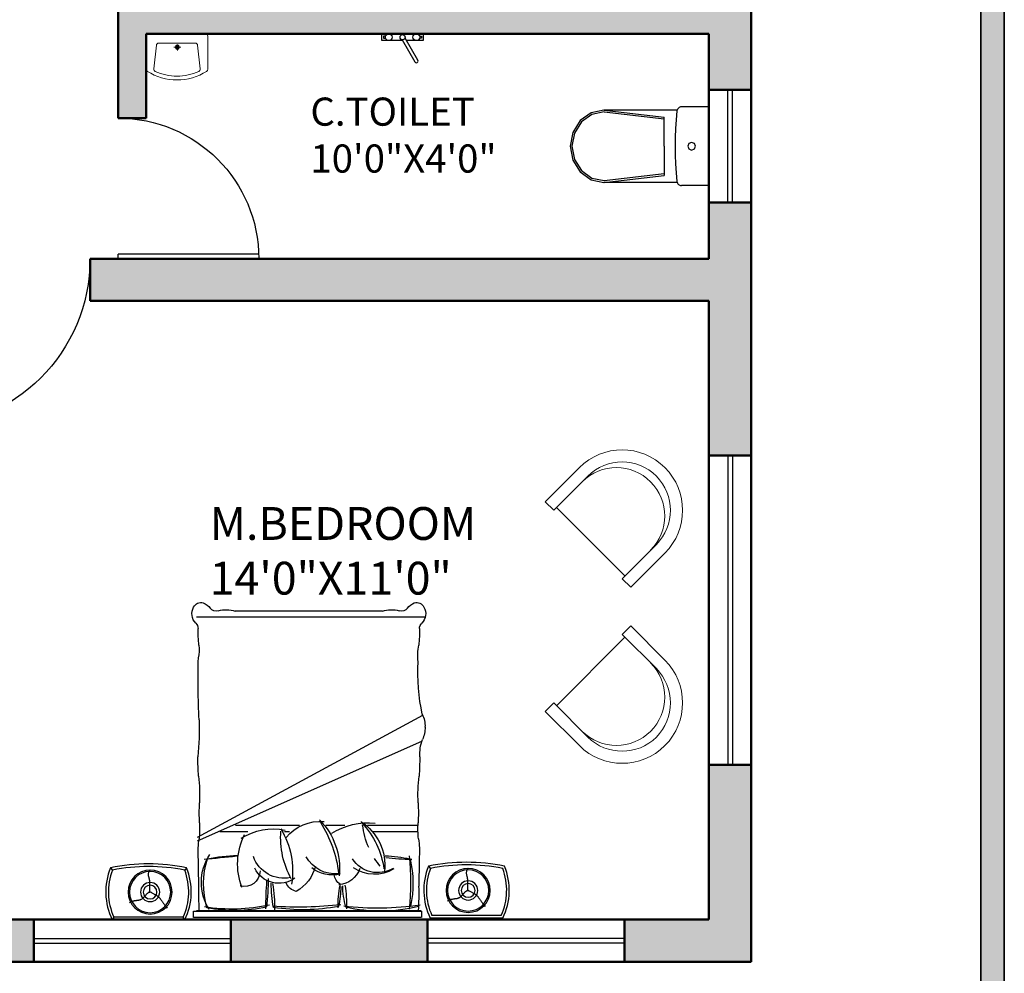
# Model space of a CAD drawing. Units: inches. Extents: x 3008 to 4088, y 1255 to 2137.
# Tile 9 of 30: x 3310 to 3520, y 1462 to 1665. Entities that reach past the tile are written whole.
import ezdxf

# ---------------------------------------------------------------- set-up
doc = ezdxf.new("R2010")
doc.units = ezdxf.units.IN
for name, color, linetype, lineweight in [('A-AREA-IDEN', 7, 'Continuous', 18), ('A-DOOR', 4, 'Continuous', 25), ('A-FLOR-FIXT', 8, 'Continuous', 18), ('A-FURN', 8, 'Continuous', 18), ('A-GLAZ', 4, 'Continuous', 25), ('A-WALL', 7, 'Continuous', 50), ('A-WALL-PATT', 8, 'Continuous', 13), ('C-PROP', 1, 'Continuous', 35), ('C-PROP-PATT', 9, 'Continuous', 13)]:
    doc.layers.add(name, color=color, linetype=linetype, lineweight=lineweight)
doc.layers.add('SANTEH', color=7, linetype='Continuous')
doc.layers.add('TEFRİŞ', color=11, linetype='Continuous')
doc.styles.get("Standard").update_dxf_attribs({"font": 'arial.ttf'})

# ---------------------------------------------------------------- blocks, each defined once
blk = doc.blocks.new('D2')
for p, q in [((1722.5, 1505.46), (1722.5, 1475.46)), ((1723.5, 1505.46), (1723.5, 1475.46)), ((1722.5, 1475.46), (1723.5, 1475.46))]:
    blk.add_line(p, q)
blk.add_arc((1722.5, 1475.46), 30, 0, 90)
blk = doc.blocks.new('D1')
for p, q in [((1805.96, 1500.36), (1805.96, 1464.36)), ((1806.96, 1500.36), (1806.96, 1464.36)), ((1805.96, 1464.36), (1806.96, 1464.36))]:
    blk.add_line(p, q)
blk.add_arc((1805.96, 1464.36), 36, 0, 90)
blk = doc.blocks.new('WC 2 Symb_109')
at = {"layer": 'SANTEH'}
for p, q in [((0, 0), (0, 380)), ((0, 380), (132.4, 380)), ((153.6, 364.9), (506.8, 364.9)), ((506.3, 364.9), (215.7, 330.9)), ((506.3, 356), (215.7, 322)), ((215.7, 190), (215.7, 330.9)), ((215.7, 190), (215.7, 49.1)), ((506.3, 24), (215.7, 58)), ((506.3, 15.1), (215.7, 49.1)), ((153.8, 15.1), (506.8, 15.1)), ((0, 0), (132.4, 0))]:
    blk.add_line(p, q, dxfattribs=at)
for points in [[(154.6, 360.1), (153.9, 364.1), (152.3, 367.9), (150.2, 371.3), (147.4, 374.3), (144.1, 376.7), (140.5, 378.5), (136.5, 379.6), (132.4, 380)], [(154.6, 19.7), (158.6, 62.1), (161.4, 104.7), (163.1, 147.3), (163.7, 189.9), (163.1, 232.5), (161.4, 275.1), (158.6, 317.7), (154.6, 360.1)], [(506.3, 24), (565.5, 36.6), (615.7, 72.6), (649.2, 126.5), (661, 190), (649.2, 253.5), (615.7, 307.4), (565.5, 343.4), (506.3, 356)], [(506.8, 15.1), (569.2, 28.4), (622.2, 66.3), (657.6, 123.1), (670, 190), (657.6, 256.9), (622.2, 313.7), (569.2, 351.6), (506.8, 364.9)], [(132.4, 0), (136.5, 0.4), (140.4, 1.5), (144.1, 3.2), (147.3, 5.6), (150.1, 8.6), (152.3, 12), (153.8, 15.7), (154.6, 19.7)]]:
    blk.add_lwpolyline(points, dxfattribs=at)
blk.add_lwpolyline([(83.6, 208.5), (70.4, 203.1), (64.9, 190), (70.4, 176.9), (83.6, 171.5), (96.8, 176.9), (102.2, 190), (96.8, 203.1)], close=True, dxfattribs=at)
blk = doc.blocks.new('Faucet - kit sink top')
at = {"layer": 'SANTEH'}
for p, q in [((-5.5, -0.75), (-5.5, -1.25)), ((-4.94278, -0.75), (-5.5, -0.75)), ((-5.5, -1.25), (-4.94278, -1.25)), ((-0.14775, -1.7441), (3.56698, -8.1782)), ((4.43301, -7.6782), (0.71828, -1.2441)), ((4.94278, -0.75), (5.5, -0.75)), ((5.5, -1.25), (4.94278, -1.25)), ((5.5, -0.75), (5.5, -1.25))]:
    blk.add_line(p, q, dxfattribs=at)
blk.add_lwpolyline([(-0.00587, -2), (-6, -2), (-6, 0), (6, 0), (6, -2), (1.15195, -2)], dxfattribs=at)
for centre, radius in [((-4, -1), 1), ((4, -1), 1), ((0, -1), 0.75)]:
    blk.add_circle(centre, radius, dxfattribs=at)
blk.add_arc((4, -7.9282), 0.5, 210, 30, dxfattribs=at)
blk = doc.blocks.new('A$C2EBB240D')
for p, q in [((0, 355.8), (0, 86.6)), ((480, 375.8), (20, 375.8)), ((500, 355.8), (500, 86.6)), ((60.8, 89.8), (82.3, 282.2)), ((250, 300), (102.1, 300)), ((250, 300), (397.9, 300)), ((439.2, 89.8), (417.7, 282.2))]:
    blk.add_line(p, q)
for points in [[(275.2, 266.4), (219.4, 266.4)], [(247.3, 238.5), (247.3, 288.9)]]:
    blk.add_lwpolyline(points)
for centre, radius, start, end in [((20, 355.8), 20, 90, 180), ((480, 355.8), 20, 0, 90), ((102.1, 280), 20, 90, 173.64284), ((247.3, 266.4), 16.7, 90, 270), ((247.3, 266.4), 10, 90, 270), ((247.3, 266.4), 16.7, 270, 90), ((247.3, 266.4), 10, 270, 90), ((397.9, 280), 20, 6.35716, 90), ((20, 86.6), 20, 180, 237.68921), ((80.7, 87.6), 20, 173.64284, 244.97956), ((419.3, 87.6), 20, 295.02044, 6.35716), ((480, 86.6), 20, 302.31079, 0), ((250, 450.3), 450.3, 237.68921, 270), ((250, 450.3), 420.3, 244.97956, 270), ((250, 450.3), 450.3, 270, 302.31079), ((250, 450.3), 420.3, 270, 295.02044)]:
    blk.add_arc(centre, radius, start, end)
blk = doc.blocks.new('12PSTG07')
at = {"color": 0, "linetype": 'ByBlock'}
for p, q in [((0, 15), (-12, 15)), ((0, 12), (0, 15)), ((-12, 12), (0, 12)), ((-1, -12), (-1, 12)), ((-12, -12), (0, -12)), ((0, -12), (0, -15)), ((0, -15), (-12, -15))]:
    blk.add_line(p, q, dxfattribs=at)
for centre, radius in [((-12, 0), 15), ((-12, 0), 12), ((-10, 0), 12)]:
    blk.add_arc(centre, radius, 90, 270, dxfattribs=at)
blk = doc.blocks.new('BED')
at = {"layer": 'TEFRİŞ'}
for p, q in [((2114.88, 1835.66), (2129.12, 1835.66)), ((2130.81, 1834.34), (2130.81, 1835.55)), ((2130.91, 1835.55), (2175.56, 1835.55)), ((2175.56, 1835.55), (2175.56, 1834.34)), ((2177.29, 1835.98), (2177.61, 1835.47)), ((2177.29, 1835.98), (2191.52, 1835.98)), ((2191.2, 1835.47), (2191.52, 1835.98)), ((2115.2, 1835.15), (2128.8, 1835.15)), ((2175.56, 1834.34), (2130.81, 1834.34)), ((2175, 1834.19), (2130.91, 1834.19)), ((2177.61, 1835.47), (2191.2, 1835.47)), ((2180.9, 1833.52), (2180.75, 1833.7)), ((2180.9, 1833.52), (2180.75, 1833.7)), ((2118.49, 1833.2), (2118.34, 1833.38)), ((2118.49, 1833.2), (2118.34, 1833.38)), ((2118.63, 1833.03), (2118.49, 1833.2)), ((2118.63, 1833.03), (2118.49, 1833.2)), ((2118.75, 1832.88), (2118.63, 1833.03)), ((2118.75, 1832.88), (2118.63, 1833.03)), ((2118.86, 1832.74), (2118.75, 1832.88)), ((2118.86, 1832.74), (2118.75, 1832.88)), ((2118.95, 1832.61), (2118.86, 1832.74)), ((2118.95, 1832.61), (2118.86, 1832.74)), ((2119.04, 1832.48), (2118.95, 1832.61)), ((2119.04, 1832.48), (2118.95, 1832.61)), ((2119.12, 1832.37), (2119.04, 1832.48)), ((2119.12, 1832.37), (2119.04, 1832.48)), ((2119.19, 1832.26), (2119.12, 1832.37)), ((2119.19, 1832.26), (2119.12, 1832.37)), ((2119.26, 1832.16), (2119.19, 1832.26)), ((2119.26, 1832.16), (2119.19, 1832.26)), ((2119.32, 1832.06), (2119.26, 1832.16)), ((2119.32, 1832.06), (2119.26, 1832.16)), ((2119.39, 1831.97), (2119.32, 1832.06)), ((2119.39, 1831.97), (2119.32, 1832.06)), ((2119.45, 1831.89), (2119.39, 1831.97)), ((2119.45, 1831.89), (2119.39, 1831.97)), ((2119.51, 1831.81), (2119.45, 1831.89)), ((2119.51, 1831.81), (2119.45, 1831.89)), ((2119.57, 1831.73), (2119.51, 1831.81)), ((2119.57, 1831.73), (2119.51, 1831.81)), ((2119.63, 1831.65), (2119.57, 1831.73)), ((2119.63, 1831.65), (2119.57, 1831.73)), ((2123.41, 1831.67), (2123.48, 1831.71)), ((2123.41, 1831.67), (2123.48, 1831.71)), ((2123.48, 1831.71), (2123.55, 1831.74)), ((2123.48, 1831.71), (2123.55, 1831.74)), ((2123.55, 1831.74), (2123.62, 1831.77)), ((2123.55, 1831.74), (2123.62, 1831.77)), ((2123.62, 1831.77), (2123.69, 1831.8)), ((2123.62, 1831.77), (2123.69, 1831.8)), ((2123.69, 1831.8), (2123.77, 1831.82)), ((2123.69, 1831.8), (2123.77, 1831.82)), ((2123.77, 1831.82), (2123.84, 1831.84)), ((2123.77, 1831.82), (2123.84, 1831.84)), ((2123.84, 1831.84), (2123.91, 1831.86)), ((2123.84, 1831.84), (2123.91, 1831.86)), ((2123.91, 1831.86), (2123.98, 1831.87)), ((2123.91, 1831.86), (2123.98, 1831.87)), ((2123.98, 1831.87), (2124.06, 1831.89)), ((2123.98, 1831.87), (2124.06, 1831.89)), ((2124.06, 1831.89), (2124.13, 1831.9)), ((2124.06, 1831.89), (2124.13, 1831.9)), ((2124.13, 1831.9), (2124.2, 1831.91)), ((2124.13, 1831.9), (2124.2, 1831.91)), ((2124.2, 1831.91), (2124.27, 1831.91)), ((2124.2, 1831.91), (2124.27, 1831.91)), ((2124.27, 1831.91), (2124.35, 1831.92)), ((2124.27, 1831.91), (2124.35, 1831.92)), ((2124.35, 1831.92), (2124.42, 1831.93)), ((2124.35, 1831.92), (2124.42, 1831.93)), ((2124.42, 1831.93), (2124.49, 1831.94)), ((2124.42, 1831.93), (2124.49, 1831.94)), ((2124.49, 1831.94), (2124.56, 1831.95)), ((2124.49, 1831.94), (2124.56, 1831.95)), ((2124.56, 1831.95), (2124.64, 1831.96)), ((2124.56, 1831.95), (2124.64, 1831.96)), ((2124.64, 1831.96), (2124.71, 1831.98)), ((2124.64, 1831.96), (2124.71, 1831.98)), ((2124.71, 1831.98), (2124.79, 1831.99)), ((2124.71, 1831.98), (2124.79, 1831.99)), ((2124.79, 1831.99), (2124.87, 1832.01)), ((2124.79, 1831.99), (2124.87, 1832.01)), ((2124.87, 1832.01), (2124.96, 1832.03)), ((2124.87, 1832.01), (2124.96, 1832.03)), ((2124.96, 1832.03), (2125.05, 1832.05)), ((2124.96, 1832.03), (2125.05, 1832.05)), ((2125.05, 1832.05), (2125.14, 1832.08)), ((2125.05, 1832.05), (2125.14, 1832.08)), ((2125.14, 1832.08), (2125.23, 1832.11)), ((2125.14, 1832.08), (2125.23, 1832.11)), ((2125.23, 1832.11), (2125.33, 1832.14)), ((2125.23, 1832.11), (2125.33, 1832.14)), ((2125.33, 1832.14), (2125.42, 1832.17)), ((2125.33, 1832.14), (2125.42, 1832.17)), ((2125.42, 1832.17), (2125.52, 1832.21)), ((2125.42, 1832.17), (2125.52, 1832.21)), ((2125.52, 1832.21), (2125.6, 1832.25)), ((2125.52, 1832.21), (2125.6, 1832.25)), ((2125.6, 1832.25), (2125.68, 1832.3)), ((2125.6, 1832.25), (2125.68, 1832.3)), ((2125.68, 1832.3), (2125.75, 1832.35)), ((2125.68, 1832.3), (2125.75, 1832.35)), ((2181.04, 1833.35), (2180.9, 1833.52)), ((2181.04, 1833.35), (2180.9, 1833.52)), ((2181.16, 1833.2), (2181.04, 1833.35)), ((2181.16, 1833.2), (2181.04, 1833.35)), ((2181.26, 1833.06), (2181.16, 1833.2)), ((2181.26, 1833.06), (2181.16, 1833.2)), ((2181.36, 1832.93), (2181.26, 1833.06)), ((2181.36, 1832.93), (2181.26, 1833.06)), ((2181.44, 1832.8), (2181.36, 1832.93)), ((2181.44, 1832.8), (2181.36, 1832.93)), ((2181.52, 1832.69), (2181.44, 1832.8)), ((2181.52, 1832.69), (2181.44, 1832.8)), ((2181.59, 1832.58), (2181.52, 1832.69)), ((2181.59, 1832.58), (2181.52, 1832.69)), ((2181.66, 1832.48), (2181.59, 1832.58)), ((2181.66, 1832.48), (2181.59, 1832.58)), ((2181.73, 1832.38), (2181.66, 1832.48)), ((2181.73, 1832.38), (2181.66, 1832.48)), ((2181.79, 1832.29), (2181.73, 1832.38)), ((2181.79, 1832.29), (2181.73, 1832.38)), ((2181.85, 1832.21), (2181.79, 1832.29)), ((2181.85, 1832.21), (2181.79, 1832.29)), ((2181.92, 1832.13), (2181.85, 1832.21)), ((2181.92, 1832.13), (2181.85, 1832.21)), ((2181.97, 1832.05), (2181.92, 1832.13)), ((2181.97, 1832.05), (2181.92, 1832.13)), ((2182.03, 1831.97), (2181.97, 1832.05)), ((2182.03, 1831.97), (2181.97, 1832.05)), ((2182.09, 1831.9), (2182.03, 1831.97)), ((2182.09, 1831.9), (2182.03, 1831.97)), ((2182.15, 1831.83), (2182.09, 1831.9)), ((2182.15, 1831.83), (2182.09, 1831.9)), ((2182.21, 1831.76), (2182.15, 1831.83)), ((2182.21, 1831.76), (2182.15, 1831.83)), ((2182.27, 1831.7), (2182.21, 1831.76)), ((2182.27, 1831.7), (2182.21, 1831.76)), ((2182.33, 1831.63), (2182.27, 1831.7)), ((2182.33, 1831.63), (2182.27, 1831.7)), ((2185.42, 1831.65), (2185.48, 1831.72)), ((2185.42, 1831.65), (2185.48, 1831.72)), ((2185.48, 1831.72), (2185.55, 1831.78)), ((2185.48, 1831.72), (2185.55, 1831.78)), ((2185.55, 1831.78), (2185.61, 1831.84)), ((2185.55, 1831.78), (2185.61, 1831.84)), ((2185.61, 1831.84), (2185.68, 1831.9)), ((2185.61, 1831.84), (2185.68, 1831.9)), ((2185.68, 1831.9), (2185.75, 1831.95)), ((2185.68, 1831.9), (2185.75, 1831.95)), ((2185.75, 1831.95), (2185.82, 1831.99)), ((2185.75, 1831.95), (2185.82, 1831.99)), ((2185.82, 1831.99), (2185.89, 1832.03)), ((2185.82, 1831.99), (2185.89, 1832.03)), ((2185.89, 1832.03), (2185.96, 1832.06)), ((2185.89, 1832.03), (2185.96, 1832.06)), ((2185.96, 1832.06), (2186.03, 1832.09)), ((2185.96, 1832.06), (2186.03, 1832.09)), ((2186.03, 1832.09), (2186.1, 1832.12)), ((2186.03, 1832.09), (2186.1, 1832.12)), ((2186.1, 1832.12), (2186.17, 1832.14)), ((2186.1, 1832.12), (2186.17, 1832.14)), ((2186.17, 1832.14), (2186.24, 1832.16)), ((2186.17, 1832.14), (2186.24, 1832.16)), ((2186.24, 1832.16), (2186.32, 1832.18)), ((2186.24, 1832.16), (2186.32, 1832.18)), ((2186.32, 1832.18), (2186.39, 1832.19)), ((2186.32, 1832.18), (2186.39, 1832.19)), ((2186.39, 1832.19), (2186.46, 1832.21)), ((2186.39, 1832.19), (2186.46, 1832.21)), ((2186.46, 1832.21), (2186.53, 1832.22)), ((2186.46, 1832.21), (2186.53, 1832.22)), ((2186.53, 1832.22), (2186.61, 1832.23)), ((2186.53, 1832.22), (2186.61, 1832.23)), ((2186.61, 1832.23), (2186.68, 1832.23)), ((2186.61, 1832.23), (2186.68, 1832.23)), ((2186.68, 1832.23), (2186.75, 1832.24)), ((2186.68, 1832.23), (2186.75, 1832.24)), ((2186.75, 1832.24), (2186.82, 1832.25)), ((2186.75, 1832.24), (2186.82, 1832.25)), ((2186.82, 1832.25), (2186.9, 1832.26)), ((2186.82, 1832.25), (2186.9, 1832.26)), ((2186.9, 1832.26), (2186.97, 1832.27)), ((2186.9, 1832.26), (2186.97, 1832.27)), ((2186.97, 1832.27), (2187.04, 1832.28)), ((2186.97, 1832.27), (2187.04, 1832.28)), ((2187.04, 1832.28), (2187.12, 1832.3)), ((2187.04, 1832.28), (2187.12, 1832.3)), ((2187.12, 1832.3), (2187.2, 1832.31)), ((2187.12, 1832.3), (2187.2, 1832.31)), ((2187.2, 1832.31), (2187.28, 1832.33)), ((2187.2, 1832.31), (2187.28, 1832.33)), ((2187.28, 1832.33), (2187.36, 1832.35)), ((2187.28, 1832.33), (2187.36, 1832.35)), ((2187.36, 1832.35), (2187.45, 1832.37)), ((2187.36, 1832.35), (2187.45, 1832.37)), ((2187.45, 1832.37), (2187.54, 1832.4)), ((2187.45, 1832.37), (2187.54, 1832.4)), ((2187.54, 1832.4), (2187.64, 1832.43)), ((2187.54, 1832.4), (2187.64, 1832.43)), ((2187.64, 1832.43), (2187.74, 1832.46)), ((2187.64, 1832.43), (2187.74, 1832.46)), ((2187.74, 1832.46), (2187.83, 1832.49)), ((2187.74, 1832.46), (2187.83, 1832.49)), ((2187.83, 1832.49), (2187.92, 1832.53)), ((2187.83, 1832.49), (2187.92, 1832.53)), ((2187.92, 1832.53), (2188.01, 1832.57)), ((2187.92, 1832.53), (2188.01, 1832.57)), ((2188.01, 1832.57), (2188.09, 1832.62)), ((2188.01, 1832.57), (2188.09, 1832.62)), ((2188.09, 1832.62), (2188.15, 1832.67)), ((2188.09, 1832.62), (2188.15, 1832.67)), ((2119.69, 1831.58), (2119.63, 1831.65)), ((2119.69, 1831.58), (2119.63, 1831.65)), ((2119.75, 1831.51), (2119.69, 1831.58)), ((2119.75, 1831.51), (2119.69, 1831.58)), ((2119.81, 1831.44), (2119.75, 1831.51)), ((2119.81, 1831.44), (2119.75, 1831.51)), ((2119.87, 1831.38), (2119.81, 1831.44)), ((2119.87, 1831.38), (2119.81, 1831.44)), ((2119.93, 1831.31), (2119.87, 1831.38)), ((2119.93, 1831.31), (2119.87, 1831.38)), ((2119.99, 1831.25), (2119.93, 1831.31)), ((2119.99, 1831.25), (2119.93, 1831.31)), ((2120.05, 1831.2), (2119.99, 1831.25)), ((2120.05, 1831.2), (2119.99, 1831.25)), ((2120.12, 1831.14), (2120.05, 1831.2)), ((2120.12, 1831.14), (2120.05, 1831.2)), ((2120.18, 1831.09), (2120.12, 1831.14)), ((2120.18, 1831.09), (2120.12, 1831.14)), ((2120.25, 1831.04), (2120.18, 1831.09)), ((2120.25, 1831.04), (2120.18, 1831.09)), ((2120.32, 1830.99), (2120.25, 1831.04)), ((2120.32, 1830.99), (2120.25, 1831.04)), ((2120.39, 1830.94), (2120.32, 1830.99)), ((2120.39, 1830.94), (2120.32, 1830.99)), ((2120.47, 1830.9), (2120.39, 1830.94)), ((2120.47, 1830.9), (2120.39, 1830.94)), ((2120.54, 1830.85), (2120.47, 1830.9)), ((2120.54, 1830.85), (2120.47, 1830.9)), ((2120.62, 1830.8), (2120.54, 1830.85)), ((2120.62, 1830.8), (2120.54, 1830.85)), ((2120.7, 1830.75), (2120.62, 1830.8)), ((2120.7, 1830.75), (2120.62, 1830.8)), ((2120.79, 1830.7), (2120.7, 1830.75)), ((2120.79, 1830.7), (2120.7, 1830.75)), ((2120.88, 1830.65), (2120.79, 1830.7)), ((2120.88, 1830.65), (2120.79, 1830.7)), ((2120.98, 1830.59), (2120.88, 1830.65)), ((2120.98, 1830.59), (2120.88, 1830.65)), ((2121.09, 1830.52), (2120.98, 1830.59)), ((2121.09, 1830.52), (2120.98, 1830.59)), ((2121.21, 1830.45), (2121.09, 1830.52)), ((2121.21, 1830.45), (2121.09, 1830.52)), ((2121.34, 1830.38), (2121.21, 1830.45)), ((2121.34, 1830.38), (2121.21, 1830.45)), ((2121.49, 1830.29), (2121.34, 1830.38)), ((2121.49, 1830.29), (2121.34, 1830.38)), ((2121.66, 1830.21), (2121.49, 1830.29)), ((2121.66, 1830.21), (2121.49, 1830.29)), ((2121.66, 1830.18), (2121.87, 1830.29)), ((2121.66, 1830.18), (2121.87, 1830.29)), ((2121.85, 1830.11), (2121.66, 1830.21)), ((2121.85, 1830.11), (2121.66, 1830.21)), ((2121.74, 1829.99), (2121.73, 1829.83)), ((2121.74, 1829.99), (2121.73, 1829.83)), ((2121.73, 1829.83), (2121.73, 1829.69)), ((2121.73, 1829.83), (2121.73, 1829.69)), ((2121.76, 1830.38), (2121.74, 1830.17)), ((2121.76, 1830.38), (2121.74, 1830.17)), ((2121.74, 1830.17), (2121.74, 1829.99)), ((2121.74, 1830.17), (2121.74, 1829.99)), ((2121.87, 1830.29), (2122.04, 1830.4)), ((2121.87, 1830.29), (2122.04, 1830.4)), ((2122.04, 1830.4), (2122.2, 1830.51)), ((2122.04, 1830.4), (2122.2, 1830.51)), ((2122.2, 1830.51), (2122.33, 1830.61)), ((2122.2, 1830.51), (2122.33, 1830.61)), ((2122.33, 1830.61), (2122.45, 1830.72)), ((2122.33, 1830.61), (2122.45, 1830.72)), ((2122.45, 1830.72), (2122.55, 1830.82)), ((2122.45, 1830.72), (2122.55, 1830.82)), ((2122.55, 1830.82), (2122.64, 1830.91)), ((2122.55, 1830.82), (2122.64, 1830.91)), ((2122.64, 1830.91), (2122.72, 1831.01)), ((2122.64, 1830.91), (2122.72, 1831.01)), ((2122.72, 1831.01), (2122.8, 1831.09)), ((2122.72, 1831.01), (2122.8, 1831.09)), ((2122.8, 1831.09), (2122.87, 1831.18)), ((2122.8, 1831.09), (2122.87, 1831.18)), ((2122.87, 1831.18), (2122.94, 1831.26)), ((2122.87, 1831.18), (2122.94, 1831.26)), ((2122.94, 1831.26), (2123.01, 1831.33)), ((2122.94, 1831.26), (2123.01, 1831.33)), ((2123.01, 1831.33), (2123.08, 1831.4)), ((2123.01, 1831.33), (2123.08, 1831.4)), ((2123.08, 1831.4), (2123.14, 1831.46)), ((2123.08, 1831.4), (2123.14, 1831.46)), ((2123.14, 1831.46), (2123.21, 1831.52)), ((2123.14, 1831.46), (2123.21, 1831.52)), ((2123.21, 1831.52), (2123.27, 1831.58)), ((2123.21, 1831.52), (2123.27, 1831.58)), ((2123.27, 1831.58), (2123.34, 1831.63)), ((2123.27, 1831.58), (2123.34, 1831.63)), ((2123.34, 1831.63), (2123.41, 1831.67)), ((2123.34, 1831.63), (2123.41, 1831.67)), ((2182.4, 1831.57), (2182.33, 1831.63)), ((2182.4, 1831.57), (2182.33, 1831.63)), ((2182.46, 1831.52), (2182.4, 1831.57)), ((2182.46, 1831.52), (2182.4, 1831.57)), ((2182.52, 1831.46), (2182.46, 1831.52)), ((2182.52, 1831.46), (2182.46, 1831.52)), ((2182.59, 1831.41), (2182.52, 1831.46)), ((2182.59, 1831.41), (2182.52, 1831.46)), ((2182.66, 1831.36), (2182.59, 1831.41)), ((2182.66, 1831.36), (2182.59, 1831.41)), ((2182.73, 1831.31), (2182.66, 1831.36)), ((2182.73, 1831.31), (2182.66, 1831.36)), ((2182.8, 1831.26), (2182.73, 1831.31)), ((2182.8, 1831.26), (2182.73, 1831.31)), ((2182.87, 1831.22), (2182.8, 1831.26)), ((2182.87, 1831.22), (2182.8, 1831.26)), ((2182.95, 1831.17), (2182.87, 1831.22)), ((2182.95, 1831.17), (2182.87, 1831.22)), ((2183.03, 1831.12), (2182.95, 1831.17)), ((2183.03, 1831.12), (2182.95, 1831.17)), ((2183.11, 1831.07), (2183.03, 1831.12)), ((2183.11, 1831.07), (2183.03, 1831.12)), ((2183.2, 1831.02), (2183.11, 1831.07)), ((2183.2, 1831.02), (2183.11, 1831.07)), ((2183.29, 1830.97), (2183.2, 1831.02)), ((2183.29, 1830.97), (2183.2, 1831.02)), ((2183.39, 1830.91), (2183.29, 1830.97)), ((2183.39, 1830.91), (2183.29, 1830.97)), ((2183.49, 1830.84), (2183.39, 1830.91)), ((2183.49, 1830.84), (2183.39, 1830.91)), ((2183.61, 1830.77), (2183.49, 1830.84)), ((2183.61, 1830.77), (2183.49, 1830.84)), ((2183.75, 1830.7), (2183.61, 1830.77)), ((2183.75, 1830.7), (2183.61, 1830.77)), ((2183.9, 1830.61), (2183.75, 1830.7)), ((2183.9, 1830.61), (2183.75, 1830.7)), ((2184.06, 1830.53), (2183.9, 1830.61)), ((2184.06, 1830.53), (2183.9, 1830.61)), ((2184.25, 1830.43), (2184.06, 1830.53)), ((2184.25, 1830.43), (2184.06, 1830.53)), ((2184.07, 1830.5), (2184.27, 1830.61)), ((2184.07, 1830.5), (2184.27, 1830.61)), ((2184.15, 1830.49), (2184.14, 1830.31)), ((2184.15, 1830.49), (2184.14, 1830.31)), ((2184.14, 1830.31), (2184.14, 1830.15)), ((2184.14, 1830.31), (2184.14, 1830.15)), ((2184.14, 1830.15), (2184.14, 1830.01)), ((2184.14, 1830.15), (2184.14, 1830.01)), ((2184.14, 1830.01), (2184.14, 1829.89)), ((2184.14, 1830.01), (2184.14, 1829.89)), ((2184.14, 1829.89), (2184.14, 1829.77)), ((2184.14, 1829.89), (2184.14, 1829.77)), ((2184.14, 1829.77), (2184.14, 1829.67)), ((2184.14, 1829.77), (2184.14, 1829.67)), ((2184.17, 1830.7), (2184.15, 1830.49)), ((2184.17, 1830.7), (2184.15, 1830.49)), ((2184.27, 1830.61), (2184.45, 1830.72)), ((2184.27, 1830.61), (2184.45, 1830.72)), ((2184.45, 1830.72), (2184.6, 1830.83)), ((2184.45, 1830.72), (2184.6, 1830.83)), ((2184.6, 1830.83), (2184.74, 1830.93)), ((2184.6, 1830.83), (2184.74, 1830.93)), ((2184.74, 1830.93), (2184.85, 1831.04)), ((2184.74, 1830.93), (2184.85, 1831.04)), ((2184.85, 1831.04), (2184.95, 1831.14)), ((2184.85, 1831.04), (2184.95, 1831.14)), ((2184.95, 1831.14), (2185.05, 1831.23)), ((2184.95, 1831.14), (2185.05, 1831.23)), ((2185.05, 1831.23), (2185.13, 1831.33)), ((2185.05, 1831.23), (2185.13, 1831.33)), ((2185.13, 1831.33), (2185.21, 1831.41)), ((2185.13, 1831.33), (2185.21, 1831.41)), ((2185.21, 1831.41), (2185.28, 1831.5)), ((2185.21, 1831.41), (2185.28, 1831.5)), ((2185.28, 1831.5), (2185.35, 1831.58)), ((2185.28, 1831.5), (2185.35, 1831.58)), ((2185.35, 1831.58), (2185.42, 1831.65)), ((2185.35, 1831.58), (2185.42, 1831.65)), ((2121.73, 1829.69), (2121.73, 1829.57)), ((2121.73, 1829.69), (2121.73, 1829.57)), ((2121.73, 1829.57), (2121.73, 1829.45)), ((2121.73, 1829.57), (2121.73, 1829.45)), ((2121.73, 1829.45), (2121.74, 1829.35)), ((2121.73, 1829.45), (2121.74, 1829.35)), ((2121.74, 1828.89), (2121.73, 1828.8)), ((2121.74, 1828.89), (2121.73, 1828.8)), ((2121.73, 1828.8), (2121.73, 1828.72)), ((2121.73, 1828.8), (2121.73, 1828.72)), ((2121.73, 1828.72), (2121.73, 1828.64)), ((2121.73, 1828.72), (2121.73, 1828.64)), ((2121.73, 1828.64), (2121.73, 1828.56)), ((2121.73, 1828.64), (2121.73, 1828.56)), ((2121.73, 1828.56), (2121.73, 1828.48)), ((2121.73, 1828.56), (2121.73, 1828.48)), ((2121.73, 1828.48), (2121.73, 1828.4)), ((2121.73, 1828.48), (2121.73, 1828.4)), ((2121.73, 1828.4), (2121.73, 1828.33)), ((2121.73, 1828.4), (2121.73, 1828.33)), ((2121.73, 1828.33), (2121.74, 1828.25)), ((2121.73, 1828.33), (2121.74, 1828.25)), ((2121.74, 1829.35), (2121.74, 1829.25)), ((2121.74, 1829.35), (2121.74, 1829.25)), ((2121.74, 1829.25), (2121.74, 1829.16)), ((2121.74, 1829.25), (2121.74, 1829.16)), ((2121.74, 1829.16), (2121.74, 1829.06)), ((2121.74, 1829.16), (2121.74, 1829.06)), ((2121.74, 1829.06), (2121.74, 1828.97)), ((2121.74, 1829.06), (2121.74, 1828.97)), ((2121.74, 1828.97), (2121.74, 1828.89)), ((2121.74, 1828.97), (2121.74, 1828.89)), ((2121.74, 1828.25), (2121.75, 1828.18)), ((2121.74, 1828.25), (2121.75, 1828.18)), ((2121.75, 1828.18), (2121.75, 1828.1)), ((2121.75, 1828.18), (2121.75, 1828.1)), ((2121.75, 1828.1), (2121.76, 1828.03)), ((2121.75, 1828.1), (2121.76, 1828.03)), ((2121.76, 1828.03), (2121.78, 1827.95)), ((2121.76, 1828.03), (2121.78, 1827.95)), ((2121.78, 1827.95), (2121.79, 1827.88)), ((2121.78, 1827.95), (2121.79, 1827.88)), ((2121.79, 1827.88), (2121.8, 1827.8)), ((2121.79, 1827.88), (2121.8, 1827.8)), ((2184.14, 1829.04), (2184.13, 1828.96)), ((2184.14, 1829.04), (2184.13, 1828.96)), ((2184.13, 1828.96), (2184.13, 1828.88)), ((2184.13, 1828.96), (2184.13, 1828.88)), ((2184.13, 1828.88), (2184.13, 1828.8)), ((2184.13, 1828.88), (2184.13, 1828.8)), ((2184.13, 1828.8), (2184.14, 1828.72)), ((2184.13, 1828.8), (2184.14, 1828.72)), ((2184.14, 1829.67), (2184.15, 1829.57)), ((2184.14, 1829.67), (2184.15, 1829.57)), ((2184.15, 1829.38), (2184.14, 1829.29)), ((2184.15, 1829.38), (2184.14, 1829.29)), ((2184.14, 1829.29), (2184.14, 1829.21)), ((2184.14, 1829.29), (2184.14, 1829.21)), ((2184.14, 1829.21), (2184.14, 1829.12)), ((2184.14, 1829.21), (2184.14, 1829.12)), ((2184.14, 1829.12), (2184.14, 1829.04)), ((2184.14, 1829.12), (2184.14, 1829.04)), ((2184.14, 1828.72), (2184.14, 1828.65)), ((2184.14, 1828.72), (2184.14, 1828.65)), ((2184.14, 1828.65), (2184.15, 1828.57)), ((2184.14, 1828.65), (2184.15, 1828.57)), ((2184.15, 1829.57), (2184.15, 1829.48)), ((2184.15, 1829.57), (2184.15, 1829.48)), ((2184.15, 1829.48), (2184.15, 1829.38)), ((2184.15, 1829.48), (2184.15, 1829.38)), ((2184.15, 1828.57), (2184.15, 1828.5)), ((2184.15, 1828.57), (2184.15, 1828.5)), ((2184.15, 1828.5), (2184.16, 1828.42)), ((2184.15, 1828.5), (2184.16, 1828.42)), ((2184.16, 1828.42), (2184.17, 1828.35)), ((2184.16, 1828.42), (2184.17, 1828.35)), ((2184.17, 1828.35), (2184.18, 1828.27)), ((2184.17, 1828.35), (2184.18, 1828.27)), ((2184.18, 1828.27), (2184.19, 1828.2)), ((2184.18, 1828.27), (2184.19, 1828.2)), ((2184.19, 1828.2), (2184.21, 1828.12)), ((2184.19, 1828.2), (2184.21, 1828.12)), ((2184.21, 1828.12), (2184.22, 1828.04)), ((2184.21, 1828.12), (2184.22, 1828.04)), ((2184.22, 1828.04), (2184.24, 1827.97)), ((2184.22, 1828.04), (2184.24, 1827.97)), ((2184.24, 1827.97), (2184.26, 1827.89)), ((2184.24, 1827.97), (2184.26, 1827.89)), ((2184.26, 1827.89), (2184.28, 1827.81)), ((2184.26, 1827.89), (2184.28, 1827.81)), ((2184.28, 1827.81), (2184.3, 1827.73)), ((2184.28, 1827.81), (2184.3, 1827.73)), ((2121.78, 1825.93), (2121.74, 1825.8)), ((2121.78, 1825.93), (2121.74, 1825.8)), ((2121.83, 1826.06), (2121.78, 1825.93)), ((2121.83, 1826.06), (2121.78, 1825.93)), ((2121.8, 1827.8), (2121.82, 1827.72)), ((2121.8, 1827.8), (2121.82, 1827.72)), ((2121.82, 1827.72), (2121.84, 1827.65)), ((2121.82, 1827.72), (2121.84, 1827.65)), ((2121.87, 1826.19), (2121.83, 1826.06)), ((2121.87, 1826.19), (2121.83, 1826.06)), ((2121.84, 1827.65), (2121.85, 1827.57)), ((2121.84, 1827.65), (2121.85, 1827.57)), ((2121.85, 1827.57), (2121.87, 1827.49)), ((2121.85, 1827.57), (2121.87, 1827.49)), ((2121.87, 1827.49), (2121.89, 1827.41)), ((2121.87, 1827.49), (2121.89, 1827.41)), ((2121.91, 1826.31), (2121.87, 1826.19)), ((2121.91, 1826.31), (2121.87, 1826.19)), ((2121.89, 1827.41), (2121.91, 1827.33)), ((2121.89, 1827.41), (2121.91, 1827.33)), ((2121.91, 1827.33), (2121.93, 1827.26)), ((2121.91, 1827.33), (2121.93, 1827.26)), ((2121.95, 1826.42), (2121.91, 1826.31)), ((2121.95, 1826.42), (2121.91, 1826.31)), ((2121.93, 1827.26), (2121.95, 1827.18)), ((2121.93, 1827.26), (2121.95, 1827.18)), ((2121.95, 1827.18), (2121.97, 1827.09)), ((2121.95, 1827.18), (2121.97, 1827.09)), ((2121.97, 1826.54), (2121.95, 1826.42)), ((2121.97, 1826.54), (2121.95, 1826.42)), ((2121.97, 1827.09), (2121.99, 1827.01)), ((2121.97, 1827.09), (2121.99, 1827.01)), ((2121.99, 1826.64), (2121.97, 1826.54)), ((2121.99, 1826.64), (2121.97, 1826.54)), ((2121.99, 1827.01), (2122, 1826.93)), ((2121.99, 1827.01), (2122, 1826.93)), ((2122, 1826.74), (2121.99, 1826.64)), ((2122, 1826.74), (2121.99, 1826.64)), ((2122, 1826.93), (2122.01, 1826.84)), ((2122, 1826.93), (2122.01, 1826.84)), ((2122.01, 1826.84), (2122, 1826.74)), ((2122.01, 1826.84), (2122, 1826.74)), ((2129.46, 1825.49), (2129.09, 1825.93)), ((2176.94, 1825.81), (2177.31, 1826.25)), ((2184.19, 1826.25), (2184.14, 1826.12)), ((2184.19, 1826.25), (2184.14, 1826.12)), ((2184.23, 1826.38), (2184.19, 1826.25)), ((2184.23, 1826.38), (2184.19, 1826.25)), ((2184.28, 1826.51), (2184.23, 1826.38)), ((2184.28, 1826.51), (2184.23, 1826.38)), ((2184.32, 1826.63), (2184.28, 1826.51)), ((2184.32, 1826.63), (2184.28, 1826.51)), ((2184.3, 1827.73), (2184.32, 1827.65)), ((2184.3, 1827.73), (2184.32, 1827.65)), ((2184.32, 1827.65), (2184.34, 1827.58)), ((2184.32, 1827.65), (2184.34, 1827.58)), ((2184.35, 1826.74), (2184.32, 1826.63)), ((2184.35, 1826.74), (2184.32, 1826.63)), ((2184.34, 1827.58), (2184.36, 1827.5)), ((2184.34, 1827.58), (2184.36, 1827.5)), ((2184.38, 1826.86), (2184.35, 1826.74)), ((2184.38, 1826.86), (2184.35, 1826.74)), ((2184.36, 1827.5), (2184.38, 1827.41)), ((2184.36, 1827.5), (2184.38, 1827.41)), ((2184.38, 1827.41), (2184.4, 1827.33)), ((2184.38, 1827.41), (2184.4, 1827.33)), ((2184.4, 1826.96), (2184.38, 1826.86)), ((2184.4, 1826.96), (2184.38, 1826.86)), ((2184.4, 1827.33), (2184.41, 1827.25)), ((2184.4, 1827.33), (2184.41, 1827.25)), ((2184.41, 1827.06), (2184.4, 1826.96)), ((2184.41, 1827.06), (2184.4, 1826.96)), ((2184.41, 1827.25), (2184.41, 1827.16)), ((2184.41, 1827.25), (2184.41, 1827.16)), ((2184.41, 1827.16), (2184.41, 1827.06)), ((2184.41, 1827.16), (2184.41, 1827.06)), ((2191.87, 1825.81), (2191.5, 1826.25)), ((2174.77, 1820.53), (2130.76, 1800.91)), ((2174.77, 1819.77), (2130.6, 1795.83)), ((2140.43, 1818.69), (2131.53, 1818.69)), ((2157.71, 1818.69), (2156.77, 1818.69)), ((2170.41, 1818.69), (2164.92, 1818.69)), ((2141.43, 1817.4), (2131.53, 1817.4)), ((2149.62, 1817.4), (2145.88, 1817.4)), ((2167.36, 1817.4), (2154.77, 1817.4)), ((2175, 1776.57), (2130.11, 1776.57)), ((2138.52, 1775.41), (2167.39, 1775.41))]:
    blk.add_line(p, q, dxfattribs=at)
for centre, radius, start, end in [((2126, 1830.19), 12.39, 153.8162, 202.314), ((2118, 1830.19), 12.39, 337.686, 26.1838), ((2188.4, 1830.51), 12.39, 153.8162, 202.314), ((2180.41, 1830.51), 12.39, 337.686, 26.1838), ((2126, 1830.19), 11.88, 155.3335, 201.0157), ((2118, 1830.19), 11.88, 338.9843, 24.6665), ((2188.4, 1830.51), 11.88, 155.3335, 201.0157), ((2180.41, 1830.51), 11.88, 338.9843, 24.6665), ((2122, 1861.35), 36.12, 258.6773, 281.3227), ((2184.41, 1861.67), 36.12, 258.6773, 281.3227), ((2122, 1861.35), 36.63, 258.2443, 281.7557), ((2184.41, 1861.67), 36.63, 258.2443, 281.7557)]:
    blk.add_arc(centre, radius, start, end, dxfattribs=at)
at = {"layer": 'TEFRİŞ', "extrusion": (0, 0, -1)}
for centre, major_axis, ratio, start_param, end_param in [((2121.68, 1830.24), (-3.05, -3.05), 1, 3.926991, 10.210176), ((2121.68, 1830.24), (2.86, -2.86), 1, 5.497787, 11.780972), ((2121.68, 1830.24), (2.86, -2.86), 1, 5.497787, 11.780972), ((2139.43, 1773.84), (-42.35, 42.35), 1, 0.646251, 0.896949), ((2206.14, 1830.73), (-52.86, -52.86), 1, 0.767743, 0.83177), ((2138.85, 1803.05), (-22.1, 22.1), 1, 0.544604, 1.006234), ((2181.61, 1828.44), (-34.39, 34.39), 1, -0.888486, -0.672463), ((2164.51, 1832.79), (-13.41, 13.41), 1, -0.974476, -0.730892), ((2155, 1761.9), (-50.65, -50.65), 1, 2.239512, 2.426533), ((2128.44, 1832.96), (-13.26, -13.26), 1, 3.889049, 4.127298), ((2154.12, 1796.61), (-26.46, 26.46), 1, 0.596409, 0.940188), ((2183.72, 1833.22), (-17, 17), 1, -0.967105, -0.749712), ((2168.35, 1789.27), (-1.33, 44.62), 0.875277, -0.163954, 0.163954), ((2087.32, 1833.96), (-52.37, 52.37), 1, 2.358049, 2.431787), ((2167.6, 1797.72), (-0.51, 36.47), 0.865194, -0.185965, 0.185965), ((2164.15, 1828.7), (-6.99, 6.99), 1, 1.789136, 2.946702), ((2156.76, 1828.98), (-11.9, -11.9), 1, 3.646453, 4.226155), ((2099.77, 1830.73), (-52.86, 52.86), 1, 2.311571, 2.373849), ((2184.09, 1830.56), (-3.05, -3.05), 1, 3.926991, 10.210176), ((2184.09, 1830.56), (2.86, -2.86), 1, 5.497787, 11.780972), ((2184.09, 1830.56), (2.86, -2.86), 1, 5.497787, 11.780972), ((2121.68, 1830.24), (1.33, -1.33), 1, 5.497787, 11.780972), ((2121.68, 1830.24), (1.33, -1.33), 1, 5.497787, 11.780972), ((2121.68, 1830.24), (0.952, -0.952), 1, 5.497787, 11.780972), ((2121.68, 1830.24), (0.952, -0.952), 1, 5.497787, 11.780972), ((2154.7, 1828.89), (-15.68, 15.68), 1, -1.00675, -0.580436), ((2127.6, 1828.81), (-13.23, 13.23), 1, 2.100388, 2.328052), ((2172.01, 1828.66), (-17.93, 17.93), 1, -0.753394, -0.598744), ((2134, 1828.8), (-18.62, 18.62), 1, 2.173461, 2.355043), ((2199.2, 1828.45), (-27.06, -27.06), 1, 0.770625, 0.917228), ((2184.09, 1830.56), (1.33, -1.33), 1, 5.497787, 11.780972), ((2184.09, 1830.56), (1.33, -1.33), 1, 5.497787, 11.780972), ((2184.09, 1830.56), (0.952, -0.952), 1, 5.497787, 11.780972), ((2184.09, 1830.56), (0.952, -0.952), 1, 5.497787, 11.780972), ((2159.55, 1823.33), (-5.81, 5.81), 1, -0.516587, 0.256776), ((2154.84, 1827.75), (-1.93, 1.93), 1, 0.997904, 1.977819), ((2166.67, 1824.96), (-2.93, 3.91), 0.760601, -0.723751, 0.723751), ((2675.38, 1815.09), (-384.79, -384.79), 1, 0.80103, 0.811711), ((2147.44, 1824.41), (-3.36, -3.36), 1, 1.11934, 2.270556), ((2145.66, 1827.01), (-1.62, 1.62), 1, 1.310976, 2.284591), ((2172, 1826.44), (-11.23, 11.23), 1, -1.332486, -0.624868), ((2158.82, 1823.55), (-3.74, -3.74), 1, 1.730792, 3.47045), ((2141.71, 1819.83), (-11.86, 11.86), 1, 1.850844, 2.42862), ((2157.83, 1821.53), (-4.47, 4.47), 1, 0.576679, 2.021689), ((2153.88, 1825.05), (-9.22, 9.22), 1, 1.994956, 2.818753), ((1630.53, 1815.09), (-384.79, 384.79), 1, 2.329881, 2.340562), ((2140.05, 1819.86), (-5.1, 5.1), 1, 0.238357, 1.390139), ((2139.42, 1820.79), (-4.21, -4.21), 1, 1.82161, 3.349145), ((2148.15, 1825.25), (-7.14, -7.14), 1, 6.061986, 7.190757), ((2154.93, 1828.48), (-11.96, 11.96), 1, -1.530302, -0.934407), ((2160.6, 1825.98), (-9.68, -9.68), 1, 0.009196, 0.886853), ((2148.35, 1820.65), (-4.63, -4.63), 1, 2.117602, 3.020837), ((2147.86, 1820.64), (-4.48, 4.48), 1, 0.665914, 1.867503), ((2170.68, 1829.67), (-16.79, 16.79), 1, -1.354718, -0.902276), ((2132.43, 1774.09), (-35.41, -35.41), 1, 2.362911, 2.464592), ((2140.17, 1862.96), (-27.99, 27.99), 1, 3.983025, 4.107469), ((2127.37, 1815.76), (-10.68, 10.68), 1, 1.657204, 1.779381), ((2165.73, 1860.69), (-26.41, -26.41), 1, 5.306413, 5.463767), ((2199.62, 1529.47), (-209.2, 209.2), 1, 0.675361, 0.697001), ((2146.08, 1822.57), (-10.5, 10.5), 1, -0.951783, -0.716225), ((2159.82, 1822.57), (-10.5, -10.5), 1, 3.857817, 4.093375), ((2111.06, 1818.12), (-14.48, 14.48), 1, 2.258605, 2.412359), ((2127.37, 1815.76), (-10.68, 10.68), 1, 1.94252, 2.248924), ((2194.85, 1818.12), (-14.48, 14.48), 1, -0.841563, -0.687809), ((2141.33, 1830.48), (-9.55, -9.55), 1, 4.941413, 5.601673), ((2150.79, 1825.18), (-6, 6), 1, 3.032122, 4.026148), ((2159.02, 1834.9), (-3.04, 16.53), 0.830169, 2.822117, 3.461068), ((2169.92, 1815.01), (-27.2, -27.2), 1, 0.734393, 0.836404), ((2135.98, 1815.01), (-27.2, -27.2), 1, 3.875985, 3.977996), ((2098.24, 1811.68), (-23.54, -23.54), 1, 3.885834, 4.043401), ((2207.66, 1811.68), (-23.54, -23.54), 1, 0.668988, 0.826555), ((2189.03, 1803.74), (-40.91, -40.91), 1, 0.789771, 0.855756), ((2116.87, 1803.74), (-40.91, 40.91), 1, 2.285836, 2.351822), ((2122.14, 1803.63), (-6.39, -6.39), 1, 3.886359, 4.265474), ((2222.76, 1798.77), (-34.16, -34.16), 1, 0.743488, 0.893627), ((2135.02, 1798.41), (-3.45, 3.45), 1, -0.831635, -0.314979), ((2135.48, 1798), (-3.77, -3.77), 1, 0.329385, 0.820948), ((2127.76, 1790.23), (-1, 12.37), 0.296708, 1.141067, 2.000525), ((2148.06, 1790.38), (-0.75, 67.37), 0.394952, 1.480524, 1.661068), ((2118.49, 1784.2), (-9.24, -9.24), 1, 3.839645, 4.088086), ((2182.27, 1782.99), (-5.52, -5.52), 1, 0.671703, 0.993321), ((2162.12, 1778.86), (-21.85, 21.85), 1, -0.78611, -0.680117), ((2143.78, 1778.86), (-21.85, 21.85), 1, 2.250913, 2.356906), ((2132.72, 1775.92), (-1.91, -1.91), 1, 0.284117, 1.557111), ((2129.83, 1778.8), (-0.986, 0.986), 1, 2.330985, 3.163296), ((2176.08, 1778.8), (-0.986, 0.986), 1, 4.690686, 5.522997), ((2173.18, 1775.92), (-1.91, -1.91), 1, 3.155278, 4.428271), ((2131.79, 1775.28), (-1.11, 1.11), 1, 3.629269, 5.067473), ((2130.83, 1777), (-2.49, -2.49), 1, 4.590984, 5.084038), ((2134.73, 1774.06), (-0.964, -0.964), 1, 1.381176, 2.701227), ((2136.75, 1781.14), (-4.24, 4.24), 1, 3.62713, 4.188813), ((2169.16, 1781.14), (-4.24, 4.24), 1, 3.665169, 4.226852), ((2171.17, 1774.06), (-0.964, -0.964), 1, 2.011162, 3.331212), ((2175.07, 1777), (-2.49, 2.49), 1, 4.34074, 4.833793), ((2174.12, 1775.28), (-1.11, 1.11), 1, 2.786508, 4.224712)]:
    blk.add_ellipse(centre, major_axis=major_axis, ratio=ratio, start_param=start_param, end_param=end_param, dxfattribs=at)

msp = doc.modelspace()

# ---------------------------------------------------------------- hatches: boundary and pattern name
at = {"layer": 'A-WALL-PATT'}
h = msp.add_hatch(color=256, dxfattribs=at)
h.dxf.hatch_style = 1
h.paths.add_polyline_path([(3102.67, 1625.97), (3093.67, 1625.97), (3093.67, 1540.97), (3102.67, 1540.97)])
h.paths.add_polyline_path([(3102.67, 1784.97), (3252.67, 1784.97), (3252.67, 1790.97), (3102.67, 1790.97), (3102.67, 1892.97), (3093.67, 1892.97), (3093.67, 1667.97), (3102.67, 1667.97)])
h.paths.add_polyline_path([(3192.67, 1943.97), (3093.67, 1943.97), (3093.67, 1934.97), (3102.67, 1934.97), (3192.67, 1934.97)])
h.paths.add_polyline_path([(3264.67, 1943.97), (3234.67, 1943.97), (3234.67, 1934.97), (3246.67, 1934.97), (3246.67, 1868.97), (3252.67, 1868.97), (3252.67, 1934.97), (3264.67, 1934.97)])
h.paths.add_polyline_path([(3330.67, 1943.97), (3288.67, 1943.97), (3288.67, 1934.97), (3300.67, 1934.97), (3300.67, 1838.97), (3246.67, 1838.97), (3246.67, 1826.97), (3252.67, 1826.97), (3252.67, 1832.97), (3306.67, 1832.97), (3306.67, 1934.97), (3330.67, 1934.97)])
h.paths.add_polyline_path([(3390.67, 1943.97), (3360.67, 1943.97), (3360.67, 1934.97), (3390.67, 1934.97)])
h.paths.add_polyline_path([(3465.67, 1943.97), (3432.67, 1943.97), (3432.67, 1934.97), (3456.67, 1934.97), (3456.67, 1883.97), (3465.67, 1883.97)])
h.paths.add_polyline_path([(3465.67, 1841.97), (3456.67, 1841.97), (3456.67, 1790.97), (3370.67, 1790.97), (3370.67, 1784.97), (3456.67, 1784.97), (3456.67, 1759.47), (3465.67, 1759.47)])
h.paths.add_polyline_path([(3465.67, 1693.47), (3456.67, 1693.47), (3456.67, 1667.97), (3330.67, 1667.97), (3330.67, 1643.97), (3336.67, 1643.97), (3336.67, 1661.97), (3456.67, 1661.97), (3456.67, 1649.97), (3465.67, 1649.97)])
h.paths.add_polyline_path([(3465.67, 1625.97), (3456.67, 1625.97), (3456.67, 1613.97), (3324.67, 1613.97), (3324.67, 1604.97), (3456.67, 1604.97), (3456.67, 1571.97), (3465.67, 1571.97)])
h.paths.add_polyline_path([(3465.67, 1505.97), (3456.67, 1505.97), (3456.67, 1472.97), (3438.67, 1472.97), (3438.67, 1463.97), (3465.67, 1463.97)])
h.paths.add_polyline_path([(3396.67, 1472.97), (3354.67, 1472.97), (3354.67, 1463.97), (3396.67, 1463.97)])
h.paths.add_polyline_path([(3312.67, 1472.97), (3288.67, 1472.97), (3288.67, 1550.97), (3282.67, 1550.97), (3282.67, 1472.97), (3270.67, 1472.97), (3270.67, 1463.97), (3312.67, 1463.97)])
h.paths.add_polyline_path([(3246.67, 1472.97), (3234.67, 1472.97), (3234.67, 1544.97), (3252.67, 1544.97), (3252.67, 1550.97), (3234.67, 1550.97), (3234.67, 1604.97), (3282.67, 1604.97), (3282.67, 1580.97), (3288.67, 1580.97), (3288.67, 1613.97), (3150.67, 1613.97), (3150.67, 1604.97), (3225.67, 1604.97), (3225.67, 1463.97), (3246.67, 1463.97)])
at = {"layer": 'C-PROP-PATT'}
h = msp.add_hatch(color=256, dxfattribs=at)
h.dxf.hatch_style = 1
h.paths.add_polyline_path([(3519.67, 2003.97), (3039.67, 2003.97), (3039.67, 1343.97), (3051.67, 1343.97), (3051.67, 1348.97), (3044.67, 1348.97), (3044.67, 1998.97), (3514.67, 1998.97), (3514.67, 1348.97), (3219.67, 1348.97), (3219.67, 1343.97), (3519.67, 1343.97)])

# ---------------------------------------------------------------- linework, layer by layer
at = {"layer": 'A-GLAZ'}
for p, q in [((3460.67, 1625.97), (3460.67, 1649.97)), ((3461.67, 1625.97), (3461.67, 1649.97)), ((3460.67, 1571.97), (3460.67, 1505.97)), ((3460.67, 1571.97), (3460.67, 1505.97)), ((3461.67, 1571.97), (3461.67, 1505.97)), ((3312.67, 1468.97), (3354.67, 1468.97)), ((3312.67, 1467.97), (3354.67, 1467.97)), ((3438.67, 1468.97), (3396.67, 1468.97)), ((3438.67, 1467.97), (3396.67, 1467.97))]:
    msp.add_line(p, q, dxfattribs=at)
at = {"layer": 'A-WALL'}
for p, q in [((3465.67, 1998.97), (3465.67, 1463.97)), ((3330.67, 1667.97), (3330.67, 1643.97)), ((3336.67, 1661.97), (3456.67, 1661.97)), ((3336.67, 1661.97), (3336.67, 1643.97)), ((3456.67, 1661.97), (3456.67, 1613.97)), ((3456.67, 1649.97), (3465.67, 1649.97)), ((3330.67, 1643.97), (3336.67, 1643.97)), ((3456.67, 1625.97), (3465.67, 1625.97)), ((3324.67, 1604.97), (3324.67, 1613.97)), ((3324.67, 1613.97), (3456.67, 1613.97)), ((3324.67, 1604.97), (3456.67, 1604.97)), ((3456.67, 1604.97), (3456.67, 1472.97)), ((3456.67, 1571.97), (3465.67, 1571.97)), ((3456.67, 1505.97), (3465.67, 1505.97)), ((3456.67, 1472.97), (3288.67, 1472.97)), ((3312.67, 1463.97), (3312.67, 1472.97)), ((3354.67, 1463.97), (3354.67, 1472.97)), ((3396.67, 1463.97), (3396.67, 1472.97)), ((3438.67, 1463.97), (3438.67, 1472.97)), ((3465.67, 1463.97), (3225.67, 1463.97))]:
    msp.add_line(p, q, dxfattribs=at)
at = {"layer": 'C-PROP'}
for p, q in [((3519.67, 2003.97), (3519.67, 1343.97)), ((3514.67, 1998.97), (3514.67, 1348.97))]:
    msp.add_line(p, q, dxfattribs=at)

# ---------------------------------------------------------------- block references
at = {"layer": 'A-DOOR', "xscale": -1}
for name, p, rotation in [('D2', (1855.21, -108.53), 270), ('D1', (1482.7, 3078.33), 180)]:
    msp.add_blockref(name, p, dxfattribs=dict(at, rotation=rotation))
at = {"layer": 'A-FLOR-FIXT'}
for name, p, xscale, yscale, zscale in [('A$C2EBB240D', (3349.77, 1652.12), -0.026211548048557, 0.026211548048557, 0.026211548048557), ('Faucet - kit sink top', (3391.33, 1661.97), 0.7356136897818673, 0.7356136897818673, 0.7356136897818673)]:
    msp.add_blockref(name, p, dxfattribs=dict(at, xscale=xscale, yscale=yscale, zscale=zscale))
at = {"layer": 'A-FLOR-FIXT', "xscale": 0.0441898926459964, "yscale": 0.0441898926459964, "zscale": 0.0441898926459964, "rotation": 180}
msp.add_blockref('WC 2 Symb_109', (3456.67, 1646.36), dxfattribs=at)
at = {"layer": 'A-FURN'}
for name, p, xscale, yscale, zscale, rotation in [('12PSTG07', (3430.86, 1553), 0.8597921787217943, 0.8597921787217943, 0.8597921787217943, 225), ('BED', (5711.32, 3468.45), 1.086875874800008, 1.086875874800008, 1.086875874800008, 180), ('12PSTG07', (3430.86, 1526.52), -0.8597921787217945, 0.8597921787217943, 0.8597921787217943, 315)]:
    msp.add_blockref(name, p, dxfattribs=dict(at, xscale=xscale, yscale=yscale, zscale=zscale, rotation=rotation))

# ---------------------------------------------------------------- texts
at = {"layer": 'A-AREA-IDEN', "attachment_point": 1}
for s, insert, char_height in [('{\\fTimes New Roman|b0|i0|c0|p18;C.TOILET\\P10\'0"X4\'0"}', (3371.67, 1648.35), 6), ('{\\fTimes New Roman|b0|i0|c0|p18;M.BEDROOM\\P14\'0"X11\'0"}', (3350.18, 1560.99), 7)]:
    msp.add_mtext_dynamic_manual_height_columns(s, width=105.6127, gutter_width=12.5, heights=[0], dxfattribs=dict(at, insert=insert, char_height=char_height))

doc.saveas('drawing.dxf')
